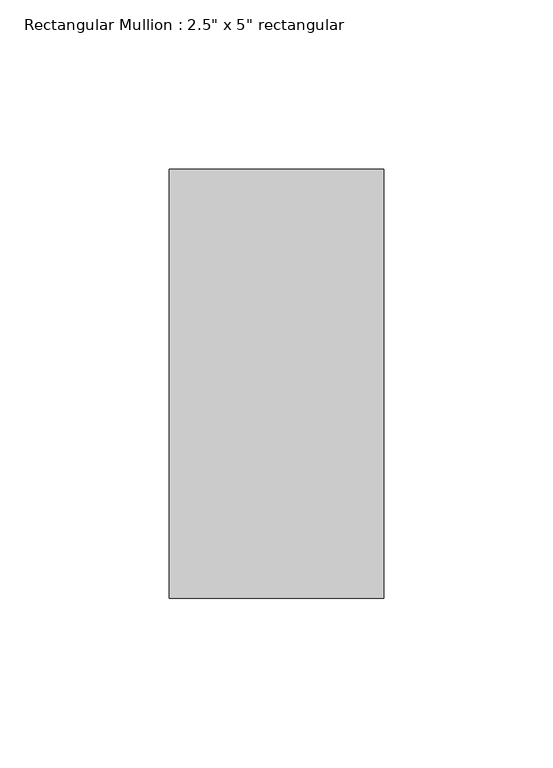
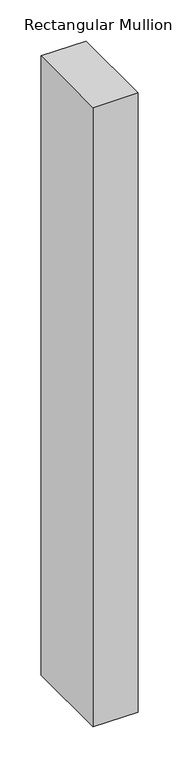
"""IFC4 building model written with IfcOpenShell, lengths in millimetres: member geometry."""

from ifc_helpers import new_model, si_unit, frame, origin, place, context, project, spatial, polyline, outline, extrude, source, transform, mapped, element, save


def member_ff82125d(model_context):
    return source(origin(), model_context, "Body", "SweptSolid", [
        extrude(outline(polyline([(0.0, 63.5), (0.0, -63.5), (-63.5, -63.5), (-63.5, 63.5), (0.0, 63.5)])), frame((0.0, 0.0, -920.75), z_axis=(0.0, 0.0, 1.0), x_axis=(1.0, 0.0, 0.0)), (0.0, 0.0, 1.0), 920.75),
    ])


if __name__ == "__main__":
    model = new_model("IFC4")
    model_context = context("Model", 3, world=origin())
    ifc_project = project(units=[si_unit("LENGTHUNIT", "METRE", prefix="MILLI")], contexts=[model_context])
    site = spatial("IfcSite", under=ifc_project)
    building = spatial("IfcBuilding", under=site)
    placement = place(None, origin())
    member_shape = member_ff82125d(model_context)
    element("IfcMember", 1, ObjectType="Rectangular Mullion : 2.5\" x 5\" rectangular", at=placement, inside=building, context=model_context, shape_type="MappedRepresentation", body=[
        mapped(member_shape, transform((0.0, 0.0, 0.0), x_axis=(1.0, 0.0, 0.0), y_axis=(0.0, 1.0, 0.0), z_axis=(0.0, 0.0, 1.0))),
    ])
    save(model, "model.ifc")

# Revit data of these elements
# Type "Rectangular Mullion : 2.5\" x 5\" rectangular"
#   built-in parameter 1007304 = 0.416667 (stored number, unit not read)
#   built-in parameter 1007301 = 0.104167 (stored number, unit not read)
#   built-in parameter 1007300 = 0.104167 (stored number, unit not read)
